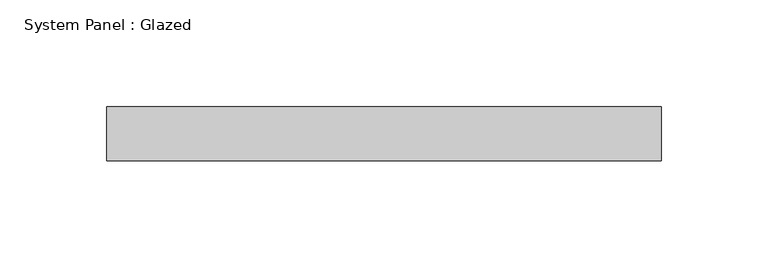
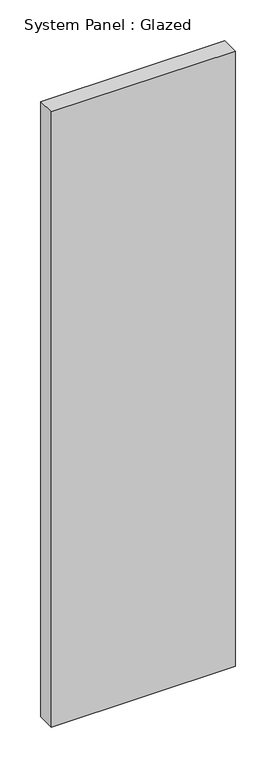
"""IFC4 building model written with IfcOpenShell, lengths in millimetres: plate geometry, System Panel : Glazed."""

from ifc_helpers import new_model, si_unit, origin, origin_with_axes, place, context, project, spatial, polyline, outline, extrude, source, transform, mapped, element, save


def system_panel_glazed_ece2a562(model_context):
    return source(origin(), model_context, "Body", "SweptSolid", [
        extrude(outline(polyline([(130.175, 19.05), (-130.175, 19.05), (-130.175, 44.45), (130.175, 44.45), (130.175, 19.05)])), origin_with_axes(), (0.0, 0.0, 1.0), 920.75),
    ])


if __name__ == "__main__":
    model = new_model("IFC4")
    model_context = context("Model", 3, world=origin())
    ifc_project = project(units=[si_unit("LENGTHUNIT", "METRE", prefix="MILLI")], contexts=[model_context])
    site = spatial("IfcSite", under=ifc_project)
    building = spatial("IfcBuilding", under=site)
    placement = place(None, origin())
    system_panel_glazed_shape = system_panel_glazed_ece2a562(model_context)
    element("IfcPlate", 1, ObjectType="System Panel : Glazed", at=placement, inside=building, context=model_context, shape_type="MappedRepresentation", body=[
        mapped(system_panel_glazed_shape, transform((0.0, 0.0, 0.0), x_axis=(1.0, 0.0, 0.0), y_axis=(0.0, 1.0, 0.0), z_axis=(0.0, 0.0, 1.0))),
    ])
    save(model, "model.ifc")

# Revit data of these elements
# Type "System Panel : Glazed"
#   Construction Type Id = "GSP4R"
#   Analytic Construction = "1/8 in Pilkington single glazing"
#   Visual Light Transmittance = 0.9
#   Solar Heat Gain Coefficient = 0.86
#   Heat Transfer Coefficient (U) = 1.18115 BTU/(h·ft²·°F)
#   Define Thermal Properties by = 1
# Element 1 (IfcPlate, "System Panel : Glazed")
#   Materials on its faces: "Glass"
# Materials
#   "Glass": class "Glass", colour RGB 0 128 192, transparency 0.75, Description = "Soda Lime Glass", Cost = 0
